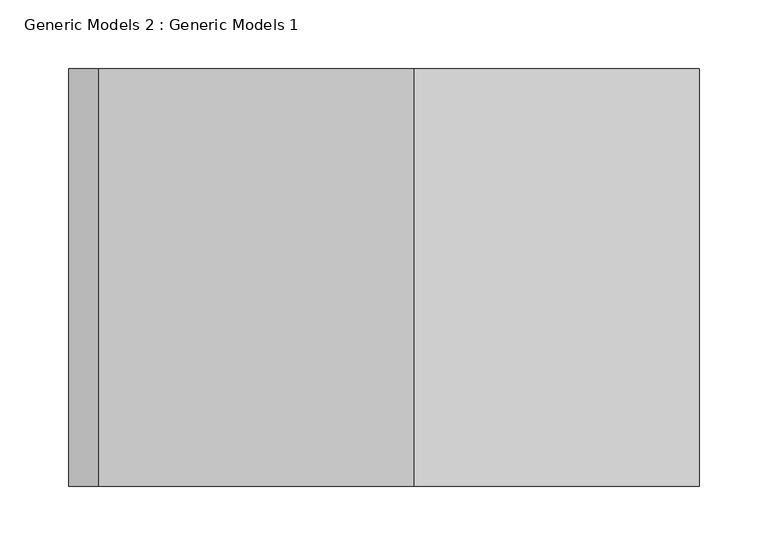
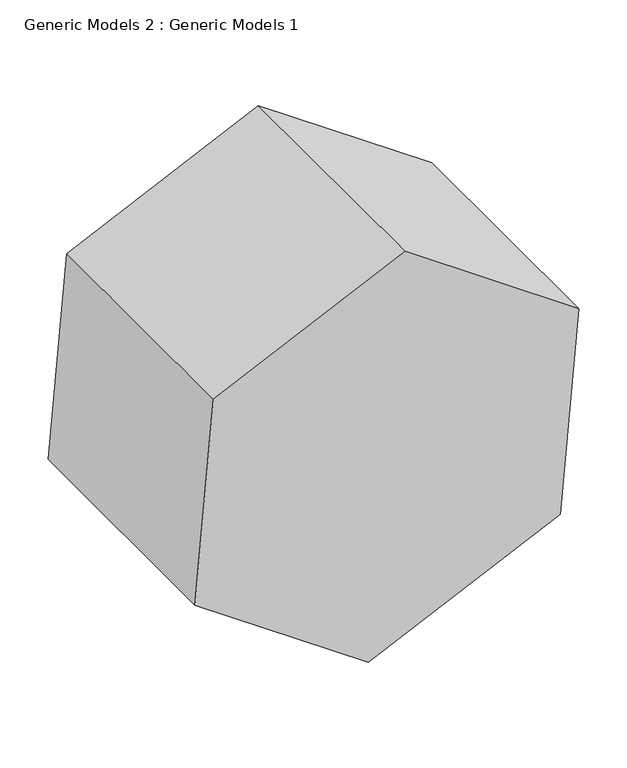
"""IFC4 building model written with IfcOpenShell, lengths in millimetres: proxy geometry, Generic Models 2 : Generic Models 1."""

from ifc_helpers import new_model, si_unit, frame, origin, place, context, project, spatial, polyline, outline, extrude, source, transform, mapped, element, save


def generic_models_2_generic_models_1_b64329ca(model_context):
    return source(origin(), model_context, "Body", "SweptSolid", [
        extrude(outline(polyline([(833.1013393, -6048.7079055), (978.7897542, -6256.7725247), (871.4447157, -6486.9747026), (618.4112624, -6509.1122613), (472.7228475, -6301.047642), (580.067886, -6070.8454641), (833.1013393, -6048.7079055)])), frame((0.0, -10720.3372434, 0.0), z_axis=(0.0, 1.0, 0.0), x_axis=(0.0, 0.0, 1.0)), (0.0, 0.0, 1.0), 304.8),
    ])


if __name__ == "__main__":
    model = new_model("IFC4")
    model_context = context("Model", 3, world=origin())
    ifc_project = project(units=[si_unit("LENGTHUNIT", "METRE", prefix="MILLI")], contexts=[model_context])
    site = spatial("IfcSite", under=ifc_project)
    building = spatial("IfcBuilding", under=site)
    placement = place(None, origin())
    generic_models_2_generic_models_1_shape = generic_models_2_generic_models_1_b64329ca(model_context)
    element("IfcBuildingElementProxy", 1, Name="Generic Models 2 : Generic Models 1", ObjectType="Generic Models 2 : Generic Models 1", at=placement, inside=building, context=model_context, shape_type="MappedRepresentation", body=[
        mapped(generic_models_2_generic_models_1_shape, transform((0.0, 0.0, 0.0), x_axis=(1.0, 0.0, 0.0), y_axis=(0.0, 1.0, 0.0), z_axis=(0.0, 0.0, 1.0))),
    ])
    save(model, "model.ifc")

# Revit data of these elements
# Element 1 (IfcBuildingElementProxy, "Generic Models 2 : Generic Models 1")
#   Materials on its faces: "Render Material 41-165-0", "Carpet (1)"
# Materials
#   "Render Material 41-165-0": colour RGB 41 165 0, transparency 0
#   "Carpet (1)": class "Carpet", colour RGB 124 80 67, transparency 0, Description = "Interior finish", Cost = 0
